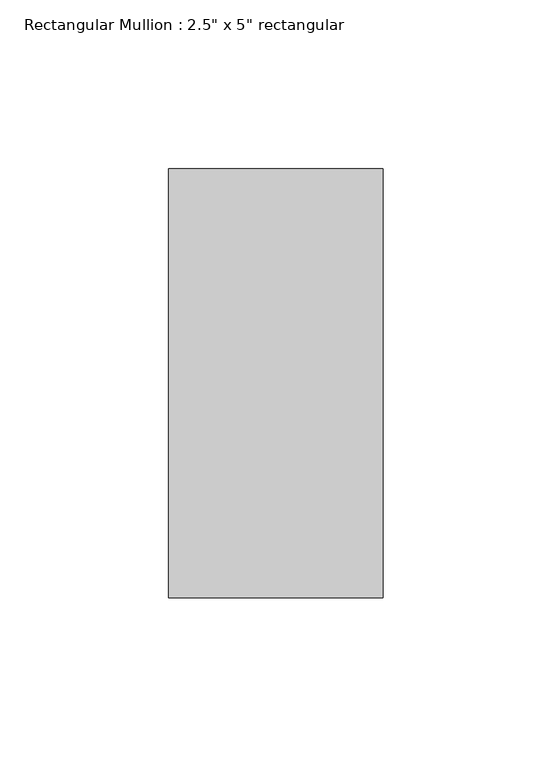
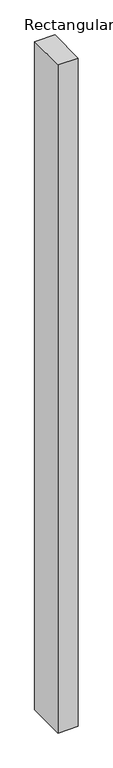
"""IFC4 building model written with IfcOpenShell, lengths in millimetres: member geometry."""

from ifc_helpers import new_model, si_unit, frame, origin, place, context, project, spatial, polyline, outline, extrude, source, transform, mapped, element, save


def member_4d884067(model_context):
    return source(origin(), model_context, "Body", "SweptSolid", [
        extrude(outline(polyline([(31.75, 63.5), (31.75, -63.5), (-31.75, -63.5), (-31.75, 63.5), (31.75, 63.5)])), frame((0.0, 0.0, -2227.7840877), z_axis=(0.0, 0.0, 1.0), x_axis=(1.0, 0.0, 0.0)), (0.0, 0.0, 1.0), 2227.7840877),
    ])


if __name__ == "__main__":
    model = new_model("IFC4")
    model_context = context("Model", 3, world=origin())
    ifc_project = project(units=[si_unit("LENGTHUNIT", "METRE", prefix="MILLI")], contexts=[model_context])
    site = spatial("IfcSite", under=ifc_project)
    building = spatial("IfcBuilding", under=site)
    placement = place(None, origin())
    member_shape = member_4d884067(model_context)
    element("IfcMember", 1, ObjectType="Rectangular Mullion : 2.5\" x 5\" rectangular", at=placement, inside=building, context=model_context, shape_type="MappedRepresentation", body=[
        mapped(member_shape, transform((0.0, 0.0, 0.0), x_axis=(1.0, 0.0, 0.0), y_axis=(0.0, 1.0, 0.0), z_axis=(0.0, 0.0, 1.0))),
    ])
    save(model, "model.ifc")

# Revit data of these elements
# Type "Rectangular Mullion : 2.5\" x 5\" rectangular"
#   built-in parameter 1007304 = 0.416667 (stored number, unit not read)
#   built-in parameter 1007301 = 0.104167 (stored number, unit not read)
#   built-in parameter 1007300 = 0.104167 (stored number, unit not read)
# Element 1 (IfcMember, "Rectangular Mullion : 2.5\" x 5\" rectangular")
#   Materials on its faces: "Aluminum"
# Materials
#   "Aluminum": class "Metal", colour RGB 247 247 247, transparency 0, Description = "Aluminum 6061", Cost = 0
